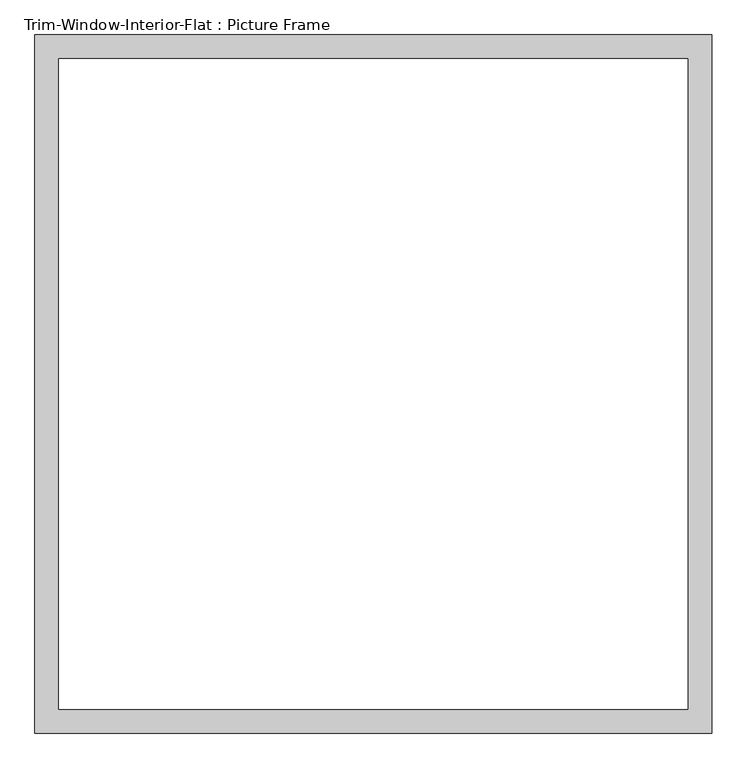
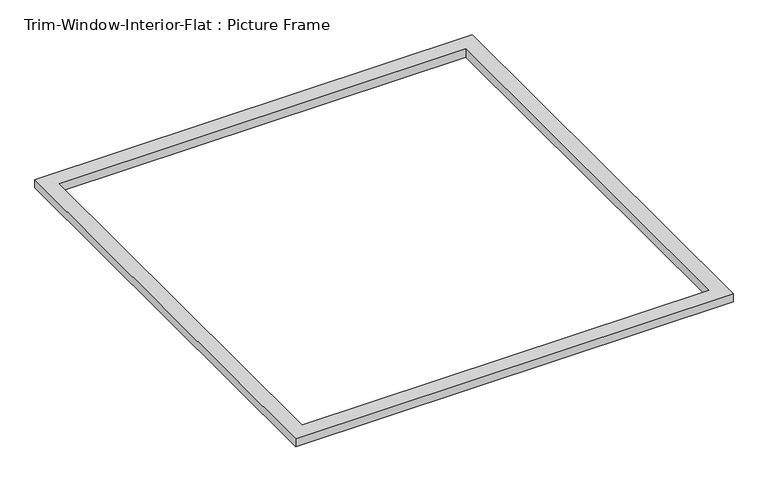
"""IFC4 building model written with IfcOpenShell, lengths in millimetres: proxy geometry, Trim-Window-Interior-Flat : Picture Frame."""

from ifc_helpers import new_model, si_unit, origin, origin_with_axes, place, context, project, spatial, polyline, outline, extrude, source, transform, mapped, element, save


def trim_window_interior_flat_picture_frame_524b5c54(model_context):
    return source(origin(), model_context, "Body", "SweptSolid", [
        extrude(outline(polyline([(806.45, 44.45), (806.45, -1619.25), (-806.45, -1619.25), (-806.45, 44.45), (806.45, 44.45)]), holes=[polyline([(749.3, -12.7), (-749.3, -12.7), (-749.3, -1562.1), (749.3, -1562.1), (749.3, -12.7)])]), origin_with_axes(), (0.0, 0.0, 1.0), 31.75),
    ])


if __name__ == "__main__":
    model = new_model("IFC4")
    model_context = context("Model", 3, world=origin())
    ifc_project = project(units=[si_unit("LENGTHUNIT", "METRE", prefix="MILLI")], contexts=[model_context])
    site = spatial("IfcSite", under=ifc_project)
    building = spatial("IfcBuilding", under=site)
    placement = place(None, origin())
    trim_window_interior_flat_picture_frame_shape = trim_window_interior_flat_picture_frame_524b5c54(model_context)
    element("IfcBuildingElementProxy", 1, Name="Trim-Window-Interior-Flat : Picture Frame", ObjectType="Trim-Window-Interior-Flat : Picture Frame", at=placement, inside=building, context=model_context, shape_type="MappedRepresentation", body=[
        mapped(trim_window_interior_flat_picture_frame_shape, transform((0.0, 0.0, 0.0), x_axis=(1.0, 0.0, 0.0), y_axis=(0.0, 1.0, 0.0), z_axis=(0.0, 0.0, 1.0))),
    ])
    save(model, "model.ifc")

# Revit data of these elements
# Type "Trim-Window-Interior-Flat : Picture Frame"
#   Trim Thickness_Picture Frame = 0' - 1 1/4"
#   Trim Width = 0' - 2 1/4"
#   Trim Thickness_with Sill = 0' - 0 3/4"
#   Sill Thickness = 0' - 1 1/4"
#   Opening Width [instance default] = 2' - 0"
#   Opening Height [instance default] = 3' - 0"
#   Default Elevation = 4' - 0"
#   Sill = no
#   Picture Frame = yes
#   Trim Material [instance default] = none
# Element 1 (IfcBuildingElementProxy, "Trim-Window-Interior-Flat : Picture Frame")
#   Opening Width = 5' - 0"
#   Opening Height = 5' - 2"
#   Trim Material = Wood - Stained
#   Materials on its faces: "Wood - Stained"
# Materials
#   "Wood - Stained": class "Wood", colour RGB 224 178 126, transparency 0, Cost = 0
